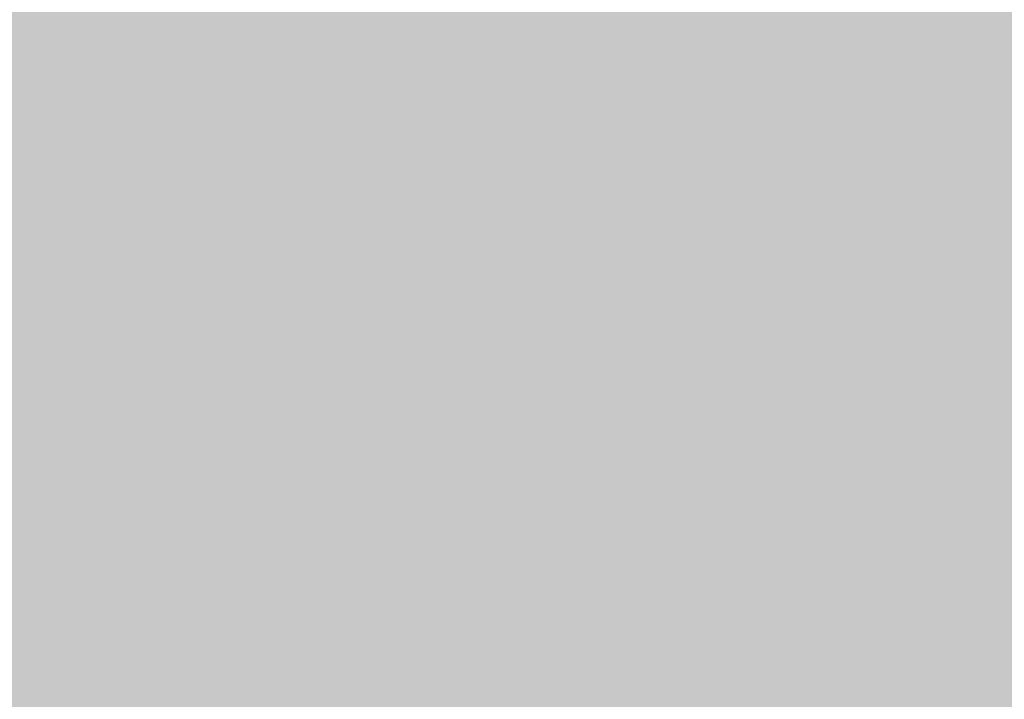
# Model space of a CAD drawing. Units: inches. Extents: x 2083 to 3317, y 1141 to 2115.
# Tile 38 of 256: x 2236.0667 to 2236.2151, y 1477.6562 to 1477.7587. Entities that reach past the tile are written whole.
import ezdxf

# ---------------------------------------------------------------- set-up
doc = ezdxf.new("R2010")
doc.units = ezdxf.units.IN
doc.layers.add('A-ANNO-DIMS', color=2, linetype='Continuous', lineweight=18)
doc.layers.add('A-WALL-PATT', color=251, linetype='Continuous', lineweight=13, true_color=0x636466)
doc.styles.get("Standard").update_dxf_attribs({"font": 'arial.ttf'})
doc.dimstyles.new('ISO-25', dxfattribs={"dimtxt": 12, "dimasz": 12, "dimexe": 1.25, "dimexo": 0.625, "dimtad": 1, "dimlunit": 3, "dimtxsty": 'Standard', "dimcen": 2.5, "dimadec": 0, "dimazin": 0, "dimtfac": 1, "dimtmove": 0, "dimatfit": 3, "dimfxl": 1, "dimarcsym": 0})

# ---------------------------------------------------------------- blocks, each defined once
blk = doc.blocks.new('*D30')
at = {"layer": 'A-ANNO-DIMS', "color": 0, "lineweight": -2, "transparency": 16777216}
for p, q in [((2240.01786, 1445.27381), (2240.01786, 1448.04553)), ((2254.32933, 1445.27381), (2254.32933, 1448.04553)), ((2228.01786, 1446.79553), (2216.01786, 1446.79553)), ((2240.01786, 1446.79553), (2254.32933, 1446.79553)), ((2266.32933, 1446.79553), (2413.76487, 1446.79553))]:
    blk.add_line(p, q, dxfattribs=at)
at = {"layer": 'A-ANNO-DIMS', "color": 0, "transparency": 16777216}
for points in [[(2228.01786, 1448.79553), (2228.01786, 1444.79553), (2240.01786, 1446.79553)], [(2266.32933, 1448.79553), (2266.32933, 1444.79553), (2254.32933, 1446.79553)]]:
    blk.add_solid(points, dxfattribs=at)
at = {"layer": 'Defpoints', "color": 0, "transparency": 16777216}
for p in [(2254.32933, 1446.79553), (2240.01786, 1444.64881), (2254.32933, 1444.64881)]:
    blk.add_point(p, dxfattribs=at)
at = {"layer": 'A-ANNO-DIMS', "color": 0, "transparency": 16777216, "insert": (2346.0471, 1453.62517), "char_height": 12, "attachment_point": 5}
blk.add_mtext('WC 1\'-2 1/2" TYP.', dxfattribs=at)
blk = doc.blocks.new('*D31')
at = {"layer": 'A-ANNO-DIMS', "color": 0, "lineweight": -2, "transparency": 16777216}
for p, q in [((2237.87114, 1456.64881), (2237.87114, 1541.91518)), ((2239.39286, 1444.64881), (2236.62114, 1444.64881)), ((2237.87114, 1431.54754), (2237.87114, 1444.64881)), ((2239.39286, 1431.54754), (2236.62114, 1431.54754)), ((2237.87114, 1419.54754), (2237.87114, 1407.54754))]:
    blk.add_line(p, q, dxfattribs=at)
at = {"layer": 'A-ANNO-DIMS', "color": 0, "transparency": 16777216}
for points in [[(2235.87114, 1456.64881), (2239.87114, 1456.64881), (2237.87114, 1444.64881)], [(2235.87114, 1419.54754), (2239.87114, 1419.54754), (2237.87114, 1431.54754)]]:
    blk.add_solid(points, dxfattribs=at)
at = {"layer": 'Defpoints', "color": 0, "transparency": 16777216}
for p in [(2237.87114, 1444.64881), (2240.01786, 1444.64881), (2240.01786, 1431.54754)]:
    blk.add_point(p, dxfattribs=at)
at = {"layer": 'A-ANNO-DIMS', "color": 0, "transparency": 16777216, "insert": (2231.21749, 1505.28199), "char_height": 12, "attachment_point": 5, "rotation": 90}
blk.add_mtext('1\'-1" TYP.', dxfattribs=at)
blk = doc.blocks.new('*D62')
at = {"layer": 'A-ANNO-DIMS', "color": 0, "lineweight": -2, "transparency": 16777216}
for p, q in [((2235.95978, 1469.38636), (2235.95978, 1522.36136)), ((2379.95978, 1469.38636), (2379.95978, 1522.36136)), ((2247.95978, 1521.11136), (2367.95978, 1521.11136))]:
    blk.add_line(p, q, dxfattribs=at)
at = {"layer": 'A-ANNO-DIMS', "color": 0, "transparency": 16777216}
for points in [[(2247.95978, 1523.11136), (2247.95978, 1519.11136), (2235.95978, 1521.11136)], [(2367.95978, 1523.11136), (2367.95978, 1519.11136), (2379.95978, 1521.11136)]]:
    blk.add_solid(points, dxfattribs=at)
at = {"layer": 'Defpoints', "color": 0, "transparency": 16777216}
for p in [(2379.95978, 1521.11136), (2235.95978, 1468.76136), (2379.95978, 1468.76136)]:
    blk.add_point(p, dxfattribs=at)
at = {"layer": 'A-ANNO-DIMS', "color": 0, "transparency": 16777216, "insert": (2307.95978, 1527.86324), "char_height": 12, "attachment_point": 5}
blk.add_mtext('12\'-0"', dxfattribs=at)

msp = doc.modelspace()

# ---------------------------------------------------------------- hatches: boundary and pattern name
at = {"layer": 'A-WALL-PATT'}
h = msp.add_hatch(color=256, dxfattribs=at)
h.dxf.hatch_style = 1
h.paths.add_polyline_path([(3126.95978, 2020.76136), (2748.95978, 2020.76136), (2604.95978, 2020.76136), (2226.95978, 2020.76136), (2226.95978, 1702.76136), (2466.95978, 1702.76136), (2466.95978, 1582.76136), (2418.95978, 1582.76136), (2418.95978, 1477.76136), (2226.95978, 1477.76136), (2226.95978, 1263.26136), (2544.95978, 1263.26136), (2544.95978, 1411.76136), (2604.95978, 1411.76136), (2685.95978, 1411.76136), (2685.95978, 1420.76136), (2604.95978, 1420.76136), (2604.95978, 1573.76136), (2604.95978, 1702.76136), (2604.95978, 2011.76136), (2748.95978, 2011.76136), (2748.95978, 1702.76136), (2862.95978, 1702.76136), (2862.95978, 1621.76136), (2871.95978, 1621.76136), (2871.95978, 1702.76136), (2883.95978, 1702.76136), (2883.95978, 1706.93946, -0.026459), (2883.95978, 1711.76136), (2757.95978, 1711.76136), (2757.95978, 1807.76136), (2787.95978, 1807.76136), (2787.95978, 1812.26136), (2757.95978, 1812.26136), (2757.95978, 2011.76136), (2877.95978, 2011.76136), (2877.95978, 1812.26136), (2847.95978, 1812.26136), (2847.95978, 1807.76136), (2889.83574, 1807.76136), (2889.83574, 1812.26136), (2882.45978, 1812.26136), (2882.45978, 2011.76136), (3117.95978, 2011.76136), (3117.95978, 1812.26136), (2937.83574, 1812.26136), (2937.83574, 1807.76136), (2995.70978, 1807.76136), (2995.70978, 1796.11767), (3000.20978, 1796.11767), (3000.20978, 1807.76136), (3117.95978, 1807.76136), (3117.95978, 1711.76136), (3000.20978, 1711.76136), (3000.20978, 1760.11767), (2998.5727, 1760.11767, -0.020711), (2995.70978, 1760.11767), (2995.70978, 1711.76136), (2931.95978, 1711.76136), (2931.95978, 1702.76136), (3126.95978, 1702.76136)])
h.paths.add_polyline_path([(2471.45978, 2011.76136), (2471.45978, 1810.01136), (2462.71694, 1810.01136), (2462.71694, 1805.51136), (2505.95978, 1805.51136), (2505.95978, 1810.01136), (2475.95978, 1810.01136), (2475.95978, 2011.76136), (2595.95978, 2011.76136), (2595.95978, 1810.01136), (2565.95978, 1810.01136), (2565.95978, 1805.51136), (2595.95978, 1805.51136), (2595.95978, 1711.76136), (2235.95978, 1711.76136), (2235.95978, 1805.51136), (2353.70978, 1805.51136), (2353.70978, 1796.05416), (2358.20978, 1796.05416), (2358.20978, 1805.51136), (2414.71694, 1805.51136), (2414.71694, 1810.01136), (2235.95978, 1810.01136), (2235.95978, 2011.76136)], flags=16)
h.paths.add_polyline_path([(2270.20473, 1994.61001), (2270.20473, 1970.61001), (2246.20473, 1970.61001), (2246.20473, 1994.61001)], flags=0)
edge = h.paths.add_edge_path(flags=0)
edge.add_ellipse((2332.02739, 1899.79818), major_axis=(-3.04299, 3.04299), ratio=0.1682525, start_angle=-161.33217, end_angle=-156.30711, ccw=False)
edge.add_ellipse((2333.08204, 1898.74353), major_axis=(-1.05465, 1.05465), ratio=0.4535321, start_angle=-123.37102, end_angle=-94.15911)
edge = h.paths.add_edge_path(flags=0)
edge.add_ellipse((2332.02739, 1968.87629), major_axis=(3.04299, 3.04299), ratio=0.1682525, start_angle=18.66783, end_angle=23.69289)
edge.add_spline(control_points=[(2332.9256, 1970.6911), (2332.22677, 1970.3361), (2330.89371, 1969.65891), (2328.41308, 1970.93214), (2327.20393, 1967.74871), (2324.7096, 1969.95559), (2322.53282, 1967.01235), (2320.01285, 1971.29581), (2317.68031, 1968.15784), (2316.04053, 1967.10205), (2315.4269, 1966.8096)], knot_values=[0, 0, 0, 0, 2.267059, 4.324559, 6.685584, 8.878641, 11.121502, 14.300359, 17.755284, 19.732645, 19.732645, 19.732645, 19.732645], degree=3, periodic=0)
edge.add_ellipse((2332.02739, 1968.87629), major_axis=(3.04299, 3.04299), ratio=0.1682525, start_angle=18.66783, end_angle=23.69289, ccw=False)
edge.add_ellipse((2333.08204, 1969.93094), major_axis=(1.05465, 1.05465), ratio=0.4535321, start_angle=56.62898, end_angle=85.84089, ccw=False)
edge = h.paths.add_edge_path(flags=0)
edge.add_spline(control_points=[(2296.42829, 1967.98791), (2293.6278, 1965.33631), (2287.70362, 1959.72709), (2299.74386, 1949.9957), (2294.53259, 1935.66853), (2290.57323, 1920.60351), (2293.39412, 1909.97369), (2296.18541, 1904.96654)], knot_values=[0.099185, 0.099185, 0.099185, 0.099185, 0.345301, 0.619822, 0.982653, 1.386093, 1.810555, 1.810555, 1.810555, 1.810555], degree=3, periodic=0)
edge.add_spline(control_points=[(2296.18541, 1904.96654), (2297.38358, 1902.6193), (2298.00097, 1901.94931), (2298.55297, 1901.46815)], knot_values=[0.006246, 0.006246, 0.006246, 0.006246, 0.055476, 0.055476, 0.055476, 0.055476], degree=3, periodic=0)
edge.add_spline(control_points=[(2298.55297, 1901.46815), (2297.25861, 1900.92322), (2295.22529, 1900.23213), (2293.06023, 1900.61421), (2292.10142, 1900.78841), (2292.08958, 1900.79057)], knot_values=[0.312835, 0.312835, 0.312835, 0.312835, 0.40178, 0.474987, 0.475903, 0.475903, 0.475903, 0.475903], degree=3, periodic=0)
edge.add_arc((2292.79365, 1904.66411), 3.93701, 215.4209, 259.69818, ccw=False)
edge.add_spline(control_points=[(2289.58531, 1902.3823), (2289.47665, 1902.53509), (2289.36848, 1902.68804), (2289.26086, 1902.84117)], knot_values=[0.102872, 0.102872, 0.102872, 0.102872, 0.116896, 0.116896, 0.116896, 0.116896], degree=3, periodic=0)
edge.add_spline(control_points=[(2289.26086, 1902.84117), (2288.6866, 1902.55019), (2287.64005, 1902.0199), (2285.88134, 1901.87395), (2283.85297, 1901.50435), (2281.71999, 1899.71054), (2278.46699, 1899.49294), (2276.15714, 1901.8832), (2272.25895, 1899.80407), (2267.77761, 1901.84318), (2262.24388, 1900.18403), (2257.41493, 1901.78206), (2254.31837, 1900.72612), (2253.17828, 1900.33734)], knot_values=[0, 0, 0, 0, 1.907977, 3.477176, 5.261074, 7.972851, 11.680248, 13.717921, 16.939592, 22.789562, 27.502503, 33.595215, 37.145618, 37.145618, 37.145618, 37.145618], degree=3, periodic=0)
edge.add_line((2253.17828, 1900.33734), (2250.24424, 1902.84117))
edge.add_line((2250.24424, 1902.84117), (2250.24424, 1965.8333))
edge.add_line((2250.24424, 1965.8333), (2253.17828, 1968.33712))
edge.add_spline(control_points=[(2253.17828, 1968.33712), (2254.31837, 1967.94835), (2257.41493, 1966.89241), (2262.24388, 1968.49043), (2267.77761, 1966.83128), (2271.52673, 1968.53722), (2273.87591, 1967.82829), (2274.2067, 1967.72764)], knot_values=[0, 0, 0, 0, 0.09018, 0.244935, 0.364644, 0.513233, 0.537855, 0.537855, 0.537855, 0.537855], degree=3, periodic=0)
edge.add_arc((2274.35289, 1963.79335), 3.93701, 72.05113, 92.12795, ccw=False)
edge.add_arc((2281.29693, 1985.23), 18.5963, 252.051134, 288.565722)
edge.add_arc((2292.31672, 1956.02888), 12.64608, 71.026788, 113.778218, ccw=False)
edge = h.paths.add_edge_path(flags=0)
edge.add_spline(control_points=[(2274.89941, 1951.85619), (2275.06616, 1951.61659), (2275.23269, 1951.37659), (2275.39799, 1951.13585)], knot_values=[1.409916, 1.409916, 1.409916, 1.409916, 1.43159, 1.43159, 1.43159, 1.43159], degree=3, periodic=0)
edge.add_spline(control_points=[(2275.39799, 1951.13585), (2275.79211, 1950.56189), (2276.17923, 1949.98377), (2276.54555, 1949.3971)], knot_values=[1.358238, 1.358238, 1.358238, 1.358238, 1.409916, 1.409916, 1.409916, 1.409916], degree=3, periodic=0)
edge.add_line((2276.54555, 1949.3971), (2277.43729, 1947.86218))
edge.add_spline(control_points=[(2277.43729, 1947.86218), (2276.30383, 1945.67311), (2274.6397, 1942.42688), (2274.63161, 1938.0939), (2272.79912, 1930.85155), (2274.35643, 1943.89705), (2275.94768, 1947.92336), (2276.54555, 1949.3971)], knot_values=[0.005632, 0.005632, 0.005632, 0.005632, 0.186014, 0.266002, 0.357087, 0.59639, 0.739732, 0.739732, 0.739732, 0.739732], degree=3, periodic=0)
edge.add_spline(control_points=[(2276.54555, 1949.3971), (2276.17923, 1949.98377), (2275.79211, 1950.56189), (2275.39799, 1951.13585)], knot_values=[1.358238, 1.358238, 1.358238, 1.358238, 1.409916, 1.409916, 1.409916, 1.409916], degree=3, periodic=0)
edge.add_spline(control_points=[(2275.39799, 1951.13585), (2274.9425, 1950.08045), (2274.20776, 1948.02527), (2273.9346, 1944.85148), (2272.46853, 1937.62749), (2273.46622, 1945.69647), (2274.70062, 1951.05947), (2274.89941, 1951.85619)], knot_values=[0.104364, 0.104364, 0.104364, 0.104364, 0.189636, 0.269624, 0.36071, 0.600013, 0.644622, 0.644622, 0.644622, 0.644622], degree=3, periodic=0)
h.paths.add_polyline_path([(2269.16751, 1963.12757, -0.357527), (2268.17063, 1960.97637, -0.092561), (2268.17063, 1939.43632, -0.357527), (2269.16751, 1937.28512, -0.357527), (2267.01631, 1938.282, -0.164785), (2254.68558, 1938.282, -0.357527), (2252.53438, 1937.28512, -0.357527), (2253.53126, 1939.43632, -0.092561), (2253.53126, 1960.97637, -0.357527), (2252.53438, 1963.12757, -0.357527), (2254.68558, 1962.13069, -0.164785), (2267.01631, 1962.13069, -0.357527)], flags=0)
h.paths.add_polyline_path([(2248.87407, 1967.8018), (2248.87407, 1957.02771), (2249.45778, 1957.02771), (2249.45778, 1911.64676), (2248.87407, 1911.64676), (2248.87407, 1900.87267), (2246.51186, 1900.87267, 0.197327), (2244.14966, 1902.45687), (2244.14966, 1966.21759, 0.197327), (2246.51186, 1967.8018)], flags=0)
h.paths.add_polyline_path([(2269.16751, 1931.38934, -0.357527), (2268.17063, 1929.23814, -0.092561), (2268.17063, 1907.6981, -0.357527), (2269.16751, 1905.54689, -0.357527), (2267.01631, 1906.54377, -0.164785), (2254.68558, 1906.54377, -0.357527), (2252.53438, 1905.54689, -0.357527), (2253.53126, 1907.6981, -0.092561), (2253.53126, 1929.23814, -0.357527), (2252.53438, 1931.38934, -0.357527), (2254.68558, 1930.39246, -0.164785), (2267.01631, 1930.39246, -0.357527)], flags=0)
edge = h.paths.add_edge_path(flags=0)
edge.add_spline(control_points=[(2276.19686, 1906.7237), (2276.16814, 1909.02893), (2276.11405, 1913.37185), (2270.59842, 1924.92498), (2273.90517, 1919.01278), (2275.92171, 1916.26206), (2275.47457, 1912.40215), (2277.25787, 1910.38062), (2276.69604, 1908.22504), (2276.64622, 1906.81302), (2276.61782, 1906.00841)], knot_values=[0, 0, 0, 0, 8.61026, 16.221274, 18.843057, 23.804898, 27.440828, 29.356102, 31.203478, 33.650687, 33.650687, 33.650687, 33.650687], degree=3, periodic=0)
edge.add_spline(control_points=[(2276.61782, 1906.00841), (2276.62331, 1905.62414), (2276.49774, 1904.62866), (2275.44178, 1903.85473), (2274.93731, 1903.08045), (2274.85908, 1902.84117)], knot_values=[0.156488, 0.156488, 0.156488, 0.156488, 0.184398, 0.231376, 0.250598, 0.250598, 0.250598, 0.250598], degree=3, periodic=0)
edge.add_line((2274.85908, 1902.84117), (2276.50598, 1902.84117))
edge.add_spline(control_points=[(2276.50598, 1902.84117), (2276.78831, 1903.08494), (2277.66507, 1904.1252), (2278.24954, 1904.34074), (2277.65387, 1908.52739), (2278.15567, 1906.22781), (2278.10046, 1905.28595), (2278.84667, 1904.06901), (2277.85679, 1903.41495), (2277.87419, 1902.99105), (2277.90356, 1902.84117)], knot_values=[0.059574, 0.059574, 0.059574, 0.059574, 0.080753, 0.103741, 0.16972, 0.176036, 0.207137, 0.240474, 0.262341, 0.27366, 0.27366, 0.27366, 0.27366], degree=3, periodic=0)
edge.add_line((2277.90356, 1902.84117), (2280.02983, 1902.84117))
edge.add_spline(control_points=[(2280.02983, 1902.84117), (2279.88822, 1903.0884), (2279.49926, 1903.98155), (2280.15228, 1905.93935), (2278.10362, 1909.65776), (2279.76239, 1907.18529), (2280.3279, 1904.87486), (2280.48511, 1903.48959), (2281.46327, 1903.24943), (2281.75834, 1902.9365), (2281.83404, 1902.84117)], knot_values=[0.013856, 0.013856, 0.013856, 0.013856, 0.034874, 0.088867, 0.107879, 0.126738, 0.158714, 0.193757, 0.217487, 0.226722, 0.226722, 0.226722, 0.226722], degree=3, periodic=0)
edge.add_spline(control_points=[(2281.83404, 1902.84117), (2281.78753, 1902.8267), (2281.64702, 1902.78299), (2281.39553, 1902.85949), (2281.08808, 1902.98524), (2280.72068, 1903.0609), (2280.33345, 1903.02573), (2280.12477, 1902.89888), (2280.02983, 1902.84117)], knot_values=[0, 0, 0, 0, 0.14413, 0.435517, 0.749276, 1.153046, 1.548371, 1.878348, 1.878348, 1.878348, 1.878348], degree=3, periodic=0)
edge.add_line((2280.02983, 1902.84117), (2277.90356, 1902.84117))
edge.add_spline(control_points=[(2277.90356, 1902.84117), (2277.89286, 1902.79586), (2277.8654, 1902.67964), (2277.60748, 1902.68748), (2277.27405, 1902.8007), (2276.83792, 1902.61977), (2276.58381, 1902.78926), (2276.50598, 1902.84117)], knot_values=[0, 0, 0, 0, 0.127189, 0.326199, 0.628009, 1.24357, 1.515331, 1.515331, 1.515331, 1.515331], degree=3, periodic=0)
edge.add_line((2276.50598, 1902.84117), (2274.85908, 1902.84117))
edge.add_spline(control_points=[(2274.85908, 1902.84117), (2274.81444, 1902.89859), (2274.72513, 1903.01345), (2274.49348, 1903.11897), (2274.24429, 1902.96054), (2273.93712, 1903.18494), (2273.61404, 1902.98314), (2273.40832, 1902.88304), (2273.32225, 1902.84117)], knot_values=[0, 0, 0, 0, 0.21843, 0.436957, 0.687977, 0.990379, 1.398396, 1.69185, 1.69185, 1.69185, 1.69185], degree=3, periodic=0)
edge.add_spline(control_points=[(2273.32225, 1902.84117), (2273.61674, 1903.44569), (2274.274, 1904.53825), (2276.02724, 1904.5737), (2276.20696, 1906.58364), (2276.19686, 1906.7237)], knot_values=[0.012227, 0.012227, 0.012227, 0.012227, 0.059472, 0.106218, 0.134458, 0.134458, 0.134458, 0.134458], degree=3, periodic=0)
h.paths.add_polyline_path([(2270.77605, 1897.78983), (2270.77605, 1873.78983), (2246.77605, 1873.78983), (2246.77605, 1897.78983)], flags=0)
h.paths.add_polyline_path([(2353.70978, 1760.00506), (2353.70978, 1760.05416), (2358.20978, 1760.05416, -0.033729)], flags=0)
h.paths.add_polyline_path([(2321.81912, 1737.52919), (2341.99533, 1737.52919, -0.414214), (2343.20327, 1736.32124), (2343.20327, 1721.0206, -0.414214), (2341.99533, 1719.81265), (2321.81912, 1719.81265, -0.414214), (2320.61117, 1721.0206), (2320.61117, 1736.32124, -0.414214)], flags=0)
h.paths.add_polyline_path([(2324.23501, 1736.32124), (2339.57944, 1736.32124, -0.414214), (2341.99533, 1733.90535), (2341.99533, 1725.44973, -0.414214), (2339.57944, 1723.03384), (2333.68059, 1723.03384), (2333.84532, 1722.04547, -0.870646), (2335.4254, 1721.82589, -0.767327), (2333.92269, 1721.42324), (2331.29102, 1721.42324, -0.767327), (2329.78832, 1721.82589, -0.870646), (2331.3684, 1722.04547), (2331.53313, 1723.03384), (2324.23501, 1723.03384, -0.414214), (2321.81912, 1725.44973), (2321.81912, 1733.90535, -0.414214)], flags=0)
h.paths.add_polyline_path([(2570.48379, 1928.61544), (2589.68379, 1928.61544), (2590.16883, 1928.61544), (2590.16883, 1904.9934), (2570.48379, 1904.9934)], flags=0)
h.paths.add_polyline_path([(2574.44732, 1927.26382, -1), (2572.82884, 1927.26382, -1)], flags=0)
h.paths.add_polyline_path([(2573.08987, 1926.94088), (2573.92503, 1927.77604), (2574.14774, 1927.55333), (2573.31258, 1926.71817)], flags=0)
h.paths.add_polyline_path([(2578.77906, 1919.72962, -1), (2571.59166, 1919.72962, -1)], flags=0)
h.paths.add_polyline_path([(2578.38536, 1919.72962, -1), (2571.98536, 1919.72962, -1)], flags=0)
h.paths.add_polyline_path([(2331.59576, 1729.47622, -1), (2333.61795, 1729.47622, -1)], flags=0)
h.paths.add_polyline_path([(2578.03423, 1927.26382, -1), (2576.41574, 1927.26382, -1)], flags=0)
h.paths.add_polyline_path([(2576.68885, 1927.53109), (2576.91156, 1927.7538), (2577.74673, 1926.91863), (2577.52402, 1926.69592)], flags=0)
h.paths.add_polyline_path([(2578.13906, 1909.85954, -1), (2572.23166, 1909.85954, -1)], flags=0)
h.paths.add_polyline_path([(2577.74536, 1909.85954, -1), (2572.62536, 1909.85954, -1)], flags=0)
h.paths.add_polyline_path([(2583.79772, 1927.26382, -1), (2582.17923, 1927.26382, -1)], flags=0)
h.paths.add_polyline_path([(2582.71865, 1927.7538), (2583.55381, 1926.91863), (2583.3311, 1926.69592), (2582.49594, 1927.53109)], flags=0)
h.paths.add_polyline_path([(2582.49594, 1927.53109), (2582.71865, 1927.7538), (2583.55381, 1926.91863), (2583.3311, 1926.69592)], flags=0)
h.paths.add_polyline_path([(2587.73906, 1920.52962, -1), (2581.83166, 1920.52962, -1)], flags=0)
h.paths.add_polyline_path([(2587.34536, 1920.52962, -1), (2582.22536, 1920.52962, -1)], flags=0)
h.paths.add_polyline_path([(2587.38462, 1927.26382, -1), (2585.76613, 1927.26382, -1)], flags=0)
h.paths.add_polyline_path([(2586.08199, 1926.98025), (2586.91716, 1927.81541), (2587.13987, 1927.5927), (2586.3047, 1926.75754)], flags=0)
h.paths.add_polyline_path([(2588.37906, 1910.65954, -1), (2581.19166, 1910.65954, -1)], flags=0)
h.paths.add_polyline_path([(2587.98536, 1910.65954, -1), (2581.58536, 1910.65954, -1)], flags=0)
h.paths.add_polyline_path([(2417.16773, 1729.4779), (2437.34394, 1729.4779, -0.414214), (2438.55188, 1728.26995), (2438.55188, 1712.96931, -0.414214), (2437.34394, 1711.76136), (2417.16773, 1711.76136, -0.414214), (2415.95978, 1712.96931), (2415.95978, 1728.26995, -0.414214)], flags=0)
h.paths.add_polyline_path([(2419.58362, 1728.26995), (2434.92805, 1728.26995, -0.414214), (2437.34394, 1725.85406), (2437.34394, 1717.39844, -0.414214), (2434.92805, 1714.98255), (2429.0292, 1714.98255), (2429.19393, 1713.99418, -0.870646), (2430.77401, 1713.7746, -0.767327), (2429.2713, 1713.37195), (2426.63963, 1713.37195, -0.767327), (2425.13693, 1713.7746, -0.870646), (2426.71701, 1713.99418), (2426.88174, 1714.98255), (2419.58362, 1714.98255, -0.414214), (2417.16773, 1717.39844), (2417.16773, 1725.85406, -0.414214)], flags=0)
h.paths.add_polyline_path([(2419.58362, 1728.26995), (2434.92805, 1728.26995, -0.414214), (2437.34394, 1725.85406), (2437.34394, 1717.39844, -0.414214), (2434.92805, 1714.98255), (2429.0292, 1714.98255), (2428.35812, 1719.00903), (2427.55282, 1719.00903), (2426.88174, 1714.98255), (2419.58362, 1714.98255, -0.414214), (2417.16773, 1717.39844), (2417.16773, 1725.85406, -0.414214)], flags=0)
h.paths.add_polyline_path([(2426.94437, 1721.42492, -1), (2428.96656, 1721.42492, -1)], flags=0)
h.paths.add_polyline_path([(2475.95978, 1702.76136), (2595.95978, 1702.76136), (2595.95978, 1582.76136), (2475.95978, 1582.76136)], flags=16)
h.paths.add_polyline_path([(2427.95978, 1573.76136), (2595.95978, 1573.76136), (2595.95978, 1468.76136), (2595.95978, 1420.76136), (2384.45978, 1420.76136), (2384.45978, 1468.76136), (2427.95978, 1468.76136)], flags=16)
h.paths.add_polyline_path([(2379.95978, 1468.76136), (2379.95978, 1420.76136), (2235.95978, 1420.76136), (2235.95978, 1468.76136)], flags=16)
h.paths.add_polyline_path([(2317.816, 1466.69577), (2337.9922, 1466.69577, -0.414214), (2339.20015, 1465.48782), (2339.20015, 1450.18718, -0.414214), (2337.9922, 1448.97923), (2317.816, 1448.97923, -0.414214), (2316.60805, 1450.18718), (2316.60805, 1465.48782, -0.414214)], flags=0)
h.paths.add_polyline_path([(2320.23189, 1465.48782), (2335.57631, 1465.48782, -0.414214), (2337.9922, 1463.07193), (2337.9922, 1454.61631, -0.414214), (2335.57631, 1452.20042), (2329.67747, 1452.20042), (2329.84219, 1451.21205, -0.870646), (2331.42228, 1450.99247, -0.767327), (2329.91957, 1450.58983), (2327.2879, 1450.58983, -0.767327), (2325.7852, 1450.99247, -0.870646), (2327.36528, 1451.21205), (2327.53001, 1452.20042), (2320.23189, 1452.20042, -0.414214), (2317.816, 1454.61631), (2317.816, 1463.07193, -0.414214)], flags=0)
h.paths.add_polyline_path([(2320.23189, 1465.48782), (2335.57631, 1465.48782, -0.414214), (2337.9922, 1463.07193), (2337.9922, 1454.61631, -0.414214), (2335.57631, 1452.20042), (2329.67747, 1452.20042), (2329.00638, 1456.22691), (2328.20109, 1456.22691), (2327.53001, 1452.20042), (2320.23189, 1452.20042, -0.414214), (2317.816, 1454.61631), (2317.816, 1463.07193, -0.414214)], flags=0)
h.paths.add_polyline_path([(2327.59264, 1458.6428, -1), (2329.61483, 1458.6428, -1)], flags=0)
h.paths.add_polyline_path([(2244.41174, 1433.34045), (2241.92094, 1433.34045, -0.414214), (2240.01786, 1435.24354), (2240.01786, 1440.95281, -0.414211), (2241.92093, 1442.8559), (2244.41174, 1442.8559, -1.976472)], flags=0)
h.paths.add_polyline_path([(2245.35689, 1434.39754, -0.414214), (2245.35689, 1441.79881, -2.144098)], flags=0)
h.paths.add_polyline_path([(2535.95978, 1416.26136), (2535.95978, 1272.26136), (2235.95978, 1272.26136), (2235.95978, 1416.26136)], flags=16)
h.paths.add_polyline_path([(2260.11956, 1384.29284), (2260.11956, 1362.03865), (2237.86537, 1362.03865), (2237.86537, 1384.29284)], flags=0)
edge = h.paths.add_edge_path(flags=0)
edge.add_line((2318.25185, 1362.0933), (2318.1458, 1362.00097))
edge.add_ellipse((2317.44512, 1360.43104), major_axis=(2.82164, 2.82164), ratio=0.1682525, start_angle=18.66783, end_angle=20.94813, ccw=False)
edge.add_ellipse((2318.42305, 1361.40897), major_axis=(0.97793, 0.97793), ratio=0.4535321, start_angle=56.62898, end_angle=70.2262, ccw=False)
edge = h.paths.add_edge_path(flags=0)
edge.add_line((2319.10737, 1295.57108), (2319.01504, 1295.67713))
edge.add_ellipse((2317.44512, 1296.37781), major_axis=(-2.82164, 2.82164), ratio=0.1682525, start_angle=-161.33217, end_angle=-159.05187, ccw=False)
edge.add_ellipse((2318.42305, 1295.39988), major_axis=(-0.97793, 0.97793), ratio=0.4535321, start_angle=-123.37102, end_angle=-109.7738)
edge = h.paths.add_edge_path(flags=0)
edge.add_spline(control_points=[(2284.21035, 1301.17022), (2284.58069, 1300.44472), (2284.89119, 1299.89202), (2285.15955, 1299.46102)], knot_values=[0.039066, 0.039066, 0.039066, 0.039066, 0.055476, 0.055476, 0.055476, 0.055476], degree=3, periodic=0)
edge.add_line((2285.15955, 1299.46102), (2284.21035, 1301.17022))
edge = h.paths.add_edge_path(flags=0)
edge.add_line((2280.41246, 1297.29801), (2283.36999, 1297.03612))
edge.add_line((2283.36999, 1297.03612), (2286.40569, 1297.92631))
edge.add_spline(control_points=[(2286.40569, 1297.92631), (2285.30549, 1297.46312), (2284.34478, 1297.12915), (2283.36999, 1297.03612)], knot_values=[0.394369, 0.394369, 0.394369, 0.394369, 0.475903, 0.475903, 0.475903, 0.475903], degree=3, periodic=0)
edge.add_spline(control_points=[(2283.36999, 1297.03612), (2283.28139, 1297.02767), (2282.31629, 1296.95734), (2281.3125, 1297.13448), (2280.42344, 1297.29602), (2280.41246, 1297.29801)], knot_values=[0.312835, 0.312835, 0.312835, 0.312835, 0.320246, 0.393453, 0.394369, 0.394369, 0.394369, 0.394369], degree=3, periodic=0)
edge = h.paths.add_edge_path(flags=0)
edge.add_line((2284.43556, 1359.60729), (2280.44629, 1355.32805))
edge.add_line((2280.44629, 1355.32805), (2279.57999, 1351.01775))
edge.add_line((2279.57999, 1351.01775), (2282.41297, 1346.58043))
edge.add_spline(control_points=[(2282.41297, 1346.58043), (2283.15333, 1345.58924), (2284.2529, 1344.0289), (2284.80104, 1342.38717), (2284.93516, 1341.80554)], knot_values=[1.240098, 1.240098, 1.240098, 1.240098, 1.332892, 1.382712, 1.382712, 1.382712, 1.382712], degree=3, periodic=0)
edge.add_spline(control_points=[(2284.93516, 1341.80554), (2285.31911, 1340.1406), (2285.23303, 1338.4092), (2284.90994, 1336.65412)], knot_values=[1.097484, 1.097484, 1.097484, 1.097484, 1.240098, 1.240098, 1.240098, 1.240098], degree=3, periodic=0)
edge.add_spline(control_points=[(2284.90994, 1336.65412), (2284.58685, 1334.89904), (2284.02675, 1333.12027), (2283.46264, 1331.36058)], knot_values=[0.95487, 0.95487, 0.95487, 0.95487, 1.097484, 1.097484, 1.097484, 1.097484], degree=3, periodic=0)
edge.add_line((2283.46264, 1331.36058), (2281.89038, 1326.15336))
edge.add_line((2281.89038, 1326.15336), (2280.75626, 1321.05609))
edge.add_line((2280.75626, 1321.05609), (2280.2992, 1316.00198))
edge.add_line((2280.2992, 1316.00198), (2280.71593, 1310.95007))
edge.add_line((2280.71593, 1310.95007), (2282.02809, 1305.97214))
edge.add_line((2282.02809, 1305.97214), (2284.21035, 1301.17022))
edge.add_spline(control_points=[(2284.21035, 1301.17022), (2283.34073, 1302.73019), (2282.6119, 1304.33649), (2282.02809, 1305.97214)], knot_values=[0.099185, 0.099185, 0.099185, 0.099185, 0.241799, 0.241799, 0.241799, 0.241799], degree=3, periodic=0)
edge.add_spline(control_points=[(2282.02809, 1305.97214), (2281.44428, 1307.60778), (2281.00549, 1309.27276), (2280.71593, 1310.95007)], knot_values=[0.241799, 0.241799, 0.241799, 0.241799, 0.384413, 0.384413, 0.384413, 0.384413], degree=3, periodic=0)
edge.add_spline(control_points=[(2280.71593, 1310.95007), (2280.43324, 1312.58761), (2280.28939, 1314.27696), (2280.29889, 1315.96203), (2280.2992, 1316.00198)], knot_values=[0.384413, 0.384413, 0.384413, 0.384413, 0.523647, 0.527028, 0.527028, 0.527028, 0.527028], degree=3, periodic=0)
edge.add_spline(control_points=[(2280.2992, 1316.00198), (2280.31233, 1317.68696), (2280.47787, 1319.36793), (2280.75626, 1321.05609)], knot_values=[0.527028, 0.527028, 0.527028, 0.527028, 0.669642, 0.669642, 0.669642, 0.669642], degree=3, periodic=0)
edge.add_spline(control_points=[(2280.75626, 1321.05609), (2281.03465, 1322.74425), (2281.42588, 1324.43961), (2281.89038, 1326.15336)], knot_values=[0.669642, 0.669642, 0.669642, 0.669642, 0.812256, 0.812256, 0.812256, 0.812256], degree=3, periodic=0)
edge.add_spline(control_points=[(2281.89038, 1326.15336), (2282.26438, 1327.53325), (2282.78787, 1329.26181), (2283.35275, 1331.01778), (2283.46264, 1331.36058)], knot_values=[0.812256, 0.812256, 0.812256, 0.812256, 0.927087, 0.95487, 0.95487, 0.95487, 0.95487], degree=3, periodic=0)
edge.add_line((2283.46264, 1331.36058), (2284.90994, 1336.65412))
edge.add_line((2284.90994, 1336.65412), (2284.93516, 1341.80554))
edge.add_line((2284.93516, 1341.80554), (2282.41297, 1346.58043))
edge.add_spline(control_points=[(2282.41297, 1346.58043), (2281.27513, 1348.10379), (2280.07845, 1349.57032), (2279.57999, 1351.01775)], knot_values=[1.382712, 1.382712, 1.382712, 1.382712, 1.525326, 1.525326, 1.525326, 1.525326], degree=3, periodic=0)
edge.add_spline(control_points=[(2279.57999, 1351.01775), (2279.44328, 1351.41472), (2279.13631, 1352.85692), (2279.73519, 1354.29039), (2280.44629, 1355.32805)], knot_values=[1.525326, 1.525326, 1.525326, 1.525326, 1.564439, 1.667941, 1.667941, 1.667941, 1.667941], degree=3, periodic=0)
edge.add_spline(control_points=[(2280.44629, 1355.32805), (2281.42611, 1356.75784), (2282.93084, 1358.18256), (2284.43556, 1359.60729)], knot_values=[1.667941, 1.667941, 1.667941, 1.667941, 1.810555, 1.810555, 1.810555, 1.810555], degree=3, periodic=0)
edge.add_arc((2280.62307, 1348.51818), 11.72618, 71.026788, 113.778218)
edge.add_arc((2270.40489, 1375.59516), 17.24357, 252.051134, 288.565722, ccw=False)
edge.add_arc((2263.96597, 1355.71785), 3.65062, 72.05113, 92.12795)
edge.add_arc((2263.96597, 1355.71785), 3.65062, 92.12795, 177.98513)
edge.add_spline(control_points=[(2260.3176, 1355.8462), (2260.26042, 1354.22067), (2260.55128, 1350.18655), (2262.99934, 1346.76625), (2264.47274, 1344.64902)], knot_values=[1.43159, 1.43159, 1.43159, 1.43159, 1.564144, 1.770695, 1.770695, 1.770695, 1.770695], degree=3, periodic=0)
edge.add_line((2264.47274, 1344.64902), (2264.93559, 1343.98253))
edge.add_spline(control_points=[(2263.80104, 1340.24811), (2263.84324, 1340.51409), (2264.06724, 1341.75647), (2264.51269, 1343.00245), (2264.93505, 1343.98108)], knot_values=[0.53657, 0.53657, 0.53657, 0.53657, 0.559349, 0.644622, 0.644622, 0.644622, 0.644622], degree=3, periodic=0)
edge.add_spline(control_points=[(2264.93505, 1343.98108), (2265.11777, 1343.71497), (2265.29888, 1343.44791), (2265.47676, 1343.17936)], knot_values=[1.384077, 1.384077, 1.384077, 1.384077, 1.409916, 1.409916, 1.409916, 1.409916], degree=3, periodic=0)
edge.add_spline(control_points=[(2265.47676, 1343.17936), (2265.65464, 1342.91082), (2265.8293, 1342.64081), (2265.99913, 1342.36881)], knot_values=[1.358238, 1.358238, 1.358238, 1.358238, 1.384077, 1.384077, 1.384077, 1.384077], degree=3, periodic=0)
edge.add_line((2265.99913, 1342.36881), (2266.82601, 1340.94555))
edge.add_spline(control_points=[(2266.82601, 1340.94555), (2268.8944, 1337.08969), (2271.39817, 1325.843), (2270.51616, 1310.56856), (2275.91938, 1301.86061), (2277.78951, 1299.19945)], knot_values=[0.116896, 0.116896, 0.116896, 0.116896, 0.472987, 1.050969, 1.313793, 1.313793, 1.313793, 1.313793], degree=3, periodic=0)
edge.add_spline(control_points=[(2277.78951, 1299.19945), (2277.83941, 1299.12845), (2277.88943, 1299.0575), (2277.93957, 1298.98658)], knot_values=[0.109884, 0.109884, 0.109884, 0.109884, 0.116896, 0.116896, 0.116896, 0.116896], degree=3, periodic=0)
edge.add_line((2277.93957, 1298.98658), (2277.78885, 1299.19911))
edge.add_spline(control_points=[(2277.78885, 1299.19911), (2277.25658, 1298.92941), (2276.28635, 1298.4379), (2275.03935, 1298.33442), (2274.38333, 1298.2389), (2274.21525, 1298.20934)], knot_values=[33.12187, 33.12187, 33.12187, 33.12187, 35.029056, 36.598255, 37.144827, 37.144827, 37.144827, 37.144827], degree=3, periodic=0)
edge.add_line((2274.21525, 1298.20934), (2273.07315, 1297.89296))
edge.add_spline(control_points=[(2273.07315, 1297.89296), (2272.32294, 1297.57978), (2271.03915, 1296.51051), (2269.24839, 1296.22606), (2268.4231, 1296.37465)], knot_values=[26.532584, 26.532584, 26.532584, 26.532584, 29.198919, 31.839101, 31.839101, 31.839101, 31.839101], degree=3, periodic=0)
edge.add_line((2268.4231, 1296.37465), (2263.8785, 1297.45753))
edge.add_spline(control_points=[(2263.8785, 1297.45753), (2263.55608, 1297.35943), (2261.86031, 1296.83869), (2260.23878, 1297.28241), (2258.93345, 1297.51646)], knot_values=[15.919551, 15.919551, 15.919551, 15.919551, 16.939592, 21.226067, 21.226067, 21.226067, 21.226067], degree=3, periodic=0)
edge.add_line((2258.93345, 1297.51646), (2254.05523, 1297.32901))
edge.add_spline(control_points=[(2254.05523, 1297.32901), (2253.75553, 1297.29582), (2252.11368, 1297.16517), (2250.46187, 1297.54422), (2249.12969, 1297.66788)], knot_values=[5.306517, 5.306517, 5.306517, 5.306517, 6.276435, 10.613034, 10.613034, 10.613034, 10.613034], degree=3, periodic=0)
edge.add_line((2249.12969, 1297.66788), (2244.33165, 1296.87776))
edge.add_line((2244.33165, 1296.87776), (2241.61103, 1299.19945))
edge.add_line((2241.61103, 1299.19945), (2241.61103, 1357.6094))
edge.add_line((2241.61103, 1357.6094), (2244.33165, 1359.9311))
edge.add_line((2244.33165, 1359.9311), (2252.72882, 1359.54269))
edge.add_spline(control_points=[(2252.72882, 1359.54269), (2252.87094, 1359.54644), (2253.30574, 1359.54817), (2253.73984, 1359.51427), (2254.03174, 1359.48243)], knot_values=[0.233291, 0.233291, 0.233291, 0.233291, 0.244935, 0.268927, 0.268927, 0.268927, 0.268927], degree=3, periodic=0)
edge.add_line((2254.03174, 1359.48243), (2259.58719, 1359.41639))
edge.add_spline(control_points=[(2259.58719, 1359.41639), (2260.67707, 1359.6285), (2262.0732, 1359.897), (2263.52369, 1359.45928), (2263.83042, 1359.36595)], knot_values=[0.422516, 0.422516, 0.422516, 0.422516, 0.513233, 0.537855, 0.537855, 0.537855, 0.537855], degree=3, periodic=0)
edge.add_arc((2263.96597, 1355.71785), 3.65062, 72.05113, 92.12795, ccw=False)
edge.add_arc((2270.40489, 1375.59516), 17.24357, 252.051134, 288.565722)
edge.add_arc((2280.62307, 1348.51818), 11.72618, 71.026788, 113.778218, ccw=False)
h.paths.add_polyline_path([(2240.34053, 1359.43471), (2240.34053, 1349.44435), (2240.88178, 1349.44435), (2240.88178, 1307.3645), (2240.34053, 1307.3645), (2240.34053, 1297.37414), (2238.15016, 1297.37414, 0.197327), (2235.95978, 1298.84311), (2235.95978, 1357.96575, 0.197327), (2238.15016, 1359.43471)], flags=0)
h.paths.add_polyline_path([(2259.15779, 1355.1005, -0.357527), (2258.23342, 1353.10578, -0.092561), (2258.23342, 1333.1326, -0.357527), (2259.15779, 1331.13788, -0.357527), (2257.16307, 1332.06225, -0.164785), (2245.7293, 1332.06225, -0.357527), (2243.73458, 1331.13788, -0.357527), (2244.65895, 1333.1326, -0.092561), (2244.65895, 1353.10578, -0.357527), (2243.73458, 1355.1005, -0.357527), (2245.7293, 1354.17613, -0.164785), (2257.16307, 1354.17613, -0.357527)], flags=0)
edge = h.paths.add_edge_path(flags=0)
edge.add_line((2265.99913, 1342.36881), (2266.82601, 1340.94555))
edge.add_line((2266.82601, 1340.94555), (2265.30756, 1337.81407))
edge.add_line((2265.30756, 1337.81407), (2264.35823, 1334.65294))
edge.add_line((2264.35823, 1334.65294), (2264.26201, 1333.7997))
edge.add_spline(control_points=[(2264.26201, 1333.7997), (2264.20836, 1333.18705), (2264.16206, 1332.36553), (2264.00714, 1331.41393), (2263.96905, 1331.20183)], knot_values=[0.464444, 0.464444, 0.464444, 0.464444, 0.516691, 0.531608, 0.531608, 0.531608, 0.531608], degree=3, periodic=0)
edge.add_spline(control_points=[(2263.96905, 1331.20183), (2263.77453, 1330.11887), (2263.42437, 1328.79084), (2263.25742, 1328.53065), (2263.23403, 1328.51461)], knot_values=[0.372682, 0.372682, 0.372682, 0.372682, 0.44885, 0.464444, 0.464444, 0.464444, 0.464444], degree=3, periodic=0)
edge.add_spline(control_points=[(2263.23403, 1328.51461), (2263.09638, 1328.42023), (2263.13117, 1329.30148), (2263.27495, 1330.61575)], knot_values=[0.280919, 0.280919, 0.280919, 0.280919, 0.372682, 0.372682, 0.372682, 0.372682], degree=3, periodic=0)
edge.add_spline(control_points=[(2263.27495, 1330.61575), (2263.41874, 1331.93002), (2263.67152, 1333.67732), (2263.96985, 1335.31503)], knot_values=[0.189157, 0.189157, 0.189157, 0.189157, 0.280919, 0.280919, 0.280919, 0.280919], degree=3, periodic=0)
edge.add_spline(control_points=[(2263.96985, 1335.31503), (2264.1005, 1336.03219), (2264.41878, 1337.62191), (2264.75485, 1338.86443), (2264.94742, 1339.49112)], knot_values=[0.097394, 0.097394, 0.097394, 0.097394, 0.137578, 0.189157, 0.189157, 0.189157, 0.189157], degree=3, periodic=0)
edge.add_spline(control_points=[(2264.94742, 1339.49112), (2265.29002, 1340.60605), (2265.64424, 1341.494), (2265.99913, 1342.36881)], knot_values=[0.005632, 0.005632, 0.005632, 0.005632, 0.097394, 0.097394, 0.097394, 0.097394], degree=3, periodic=0)
h.paths.add_polyline_path([(2259.15779, 1325.67097, -0.357527), (2258.23342, 1323.67625, -0.092561), (2258.23342, 1303.70307, -0.357527), (2259.15779, 1301.70835, -0.357527), (2257.16307, 1302.63272, -0.164785), (2245.7293, 1302.63272, -0.357527), (2243.73458, 1301.70835, -0.357527), (2244.65895, 1303.70307, -0.092561), (2244.65895, 1323.67625, -0.357527), (2243.73458, 1325.67097, -0.357527), (2245.7293, 1324.74661, -0.164785), (2257.16307, 1324.74661, -0.357527)], flags=0)
edge = h.paths.add_edge_path(flags=0)
edge.add_spline(control_points=[(2261.70894, 1317.31142), (2261.67948, 1317.41758), (2261.76186, 1317.38853), (2262.49074, 1316.08987), (2262.96218, 1315.3009)], knot_values=[14.955861, 14.955861, 14.955861, 14.955861, 16.221274, 18.694826, 18.694826, 18.694826, 18.694826], degree=3, periodic=0)
edge.add_spline(control_points=[(2262.96218, 1315.3009), (2262.99044, 1315.25362), (2263.7021, 1314.06738), (2264.34898, 1313.12715), (2264.73005, 1312.16415)], knot_values=[18.694826, 18.694826, 18.694826, 18.694826, 18.843057, 22.433791, 22.433791, 22.433791, 22.433791], degree=3, periodic=0)
edge.add_spline(control_points=[(2264.73005, 1312.16415), (2264.87556, 1311.79644), (2265.17687, 1310.76981), (2265.14307, 1309.55926), (2265.24774, 1308.82419)], knot_values=[22.433791, 22.433791, 22.433791, 22.433791, 23.804898, 26.172756, 26.172756, 26.172756, 26.172756], degree=3, periodic=0)
edge.add_line((2265.24774, 1308.82419), (2265.85077, 1307.17189))
edge.add_spline(control_points=[(2265.85077, 1307.17189), (2266.06502, 1306.82168), (2266.38439, 1306.33225), (2266.4244, 1305.78055), (2266.42037, 1305.61122)], knot_values=[28.062562, 28.062562, 28.062562, 28.062562, 29.356102, 29.911721, 29.911721, 29.911721, 29.911721], degree=3, periodic=0)
edge.add_spline(control_points=[(2266.42037, 1305.61122), (2266.41612, 1305.43259), (2266.394, 1305.25), (2266.36478, 1305.06586)], knot_values=[29.911721, 29.911721, 29.911721, 29.911721, 30.497837, 30.497837, 30.497837, 30.497837], degree=3, periodic=0)
edge.add_line((2266.36478, 1305.06586), (2266.06615, 1302.1363))
edge.add_spline(control_points=[(2266.06615, 1302.1363), (2266.07124, 1301.77998), (2265.99808, 1301.19998), (2265.66327, 1300.75896), (2265.50891, 1300.58588)], knot_values=[0.156488, 0.156488, 0.156488, 0.156488, 0.184398, 0.203543, 0.203543, 0.203543, 0.203543], degree=3, periodic=0)
edge.add_line((2265.50891, 1300.58588), (2264.43534, 1299.19945))
edge.add_line((2264.43534, 1299.19945), (2265.96244, 1299.19945))
edge.add_line((2265.96244, 1299.19945), (2267.33599, 1301.17528))
edge.add_line((2267.33599, 1301.17528), (2267.31167, 1301.98624))
edge.add_spline(control_points=[(2267.31167, 1301.98624), (2267.26111, 1302.8624), (2267.16021, 1303.73713), (2267.27149, 1303.3259)], knot_values=[0.126229, 0.126229, 0.126229, 0.126229, 0.166617, 0.166617, 0.166617, 0.166617], degree=3, periodic=0)
edge.add_spline(control_points=[(2267.27149, 1303.3259), (2267.28003, 1303.2943), (2267.30979, 1303.17537), (2267.37345, 1302.88361), (2267.40612, 1302.68283), (2267.41793, 1302.60103)], knot_values=[0.166617, 0.166617, 0.166617, 0.166617, 0.16972, 0.176036, 0.180765, 0.180765, 0.180765, 0.180765], degree=3, periodic=0)
edge.add_spline(control_points=[(2267.74389, 1300.9875), (2267.68758, 1301.15094), (2267.48052, 1301.65666), (2267.48375, 1302.14479), (2267.41793, 1302.60103)], knot_values=[0.180765, 0.180765, 0.180765, 0.180765, 0.193767, 0.220139, 0.220139, 0.220139, 0.220139], degree=3, periodic=0)
edge.add_line((2267.41793, 1302.60103), (2267.74389, 1300.9875))
edge.add_spline(control_points=[(2267.74389, 1300.9875), (2267.83196, 1300.73188), (2267.93202, 1300.3099), (2267.55484, 1299.97452), (2267.42937, 1299.82921)], knot_values=[0.220139, 0.220139, 0.220139, 0.220139, 0.240474, 0.25489, 0.25489, 0.25489, 0.25489], degree=3, periodic=0)
edge.add_line((2267.42937, 1299.82921), (2267.25836, 1299.19945))
edge.add_line((2267.25836, 1299.19945), (2269.22996, 1299.19945))
edge.add_spline(control_points=[(2269.22996, 1299.19945), (2269.09865, 1299.42869), (2268.84277, 1300.01625), (2269.01157, 1300.91592), (2268.9468, 1301.66074)], knot_values=[0.013856, 0.013856, 0.013856, 0.013856, 0.034874, 0.067073, 0.067073, 0.067073, 0.067073], degree=3, periodic=0)
edge.add_line((2268.9468, 1301.66074), (2268.43158, 1303.60311))
edge.add_spline(control_points=[(2268.43158, 1303.60311), (2268.1756, 1304.19237), (2267.59621, 1305.2513), (2268.0407, 1304.62321), (2268.25139, 1304.28242)], knot_values=[0.090155, 0.090155, 0.090155, 0.090155, 0.107879, 0.120289, 0.120289, 0.120289, 0.120289], degree=3, periodic=0)
edge.add_spline(control_points=[(2268.25139, 1304.28242), (2268.36088, 1304.10533), (2269.05775, 1302.91798), (2269.38269, 1301.59042), (2269.52141, 1300.77593), (2269.57522, 1300.55578)], knot_values=[0.120289, 0.120289, 0.120289, 0.120289, 0.126738, 0.158714, 0.173506, 0.173506, 0.173506, 0.173506], degree=3, periodic=0)
edge.add_line((2269.57522, 1300.55578), (2270.6858, 1299.42126))
edge.add_spline(control_points=[(2270.6858, 1299.42126), (2270.76722, 1299.35725), (2270.83785, 1299.2814), (2270.90292, 1299.19945)], knot_values=[0.21816, 0.21816, 0.21816, 0.21816, 0.226722, 0.226722, 0.226722, 0.226722], degree=3, periodic=0)
edge.add_line((2270.9372, 1299.19291), (2270.90292, 1299.19945))
edge.add_spline(control_points=[(2270.90292, 1299.19945), (2270.85981, 1299.18603), (2270.72951, 1299.1455), (2270.49631, 1299.21644), (2270.27166, 1299.30832), (2270.12102, 1299.34796), (2270.06334, 1299.35956)], knot_values=[0.939174, 0.939174, 0.939174, 0.939174, 1.083304, 1.374691, 1.68845, 1.878348, 1.878348, 1.878348, 1.878348], degree=3, periodic=0)
edge.add_line((2270.06334, 1299.35956), (2269.22996, 1299.19945))
edge.add_line((2269.22996, 1299.19945), (2267.25836, 1299.19945))
edge.add_spline(control_points=[(2267.25836, 1299.19945), (2267.24843, 1299.15743), (2267.22297, 1299.04967), (2266.98382, 1299.05694), (2266.80921, 1299.11623), (2266.6769, 1299.10909), (2266.63653, 1299.10481)], knot_values=[0.757665, 0.757665, 0.757665, 0.757665, 0.884854, 1.083864, 1.385675, 1.515331, 1.515331, 1.515331, 1.515331], degree=3, periodic=0)
edge.add_spline(control_points=[(2266.63653, 1299.10481), (2266.48522, 1299.08879), (2266.23581, 1299.01712), (2266.03461, 1299.15132), (2265.96244, 1299.19945)], knot_values=[0, 0, 0, 0, 0.485905, 0.757665, 0.757665, 0.757665, 0.757665], degree=3, periodic=0)
edge.add_line((2265.96244, 1299.19945), (2264.43534, 1299.19945))
edge.add_line((2264.43534, 1299.19945), (2263.85844, 1299.36712))
edge.add_spline(control_points=[(2263.85844, 1299.36712), (2263.81894, 1299.37091), (2263.77953, 1299.38572), (2263.74013, 1299.4015)], knot_values=[0.845925, 0.845925, 0.845925, 0.845925, 0.978627, 0.978627, 0.978627, 0.978627], degree=3, periodic=0)
edge.add_line((2263.72179, 1299.39643), (2263.01031, 1299.19945))
edge.add_spline(control_points=[(2263.01031, 1299.19945), (2263.24579, 1299.68286), (2263.50603, 1300.12811), (2263.87349, 1300.40803)], knot_values=[0.012227, 0.012227, 0.012227, 0.012227, 0.052971, 0.052971, 0.052971, 0.052971], degree=3, periodic=0)
edge.add_spline(control_points=[(2263.87349, 1300.40803), (2263.93213, 1300.4527), (2264.08424, 1300.55298), (2264.25519, 1300.62422), (2264.35969, 1300.66475)], knot_values=[0.052971, 0.052971, 0.052971, 0.052971, 0.059472, 0.069086, 0.069086, 0.069086, 0.069086], degree=3, periodic=0)
edge.add_line((2264.35969, 1300.66475), (2265.1419, 1301.07777))
edge.add_line((2265.1419, 1301.07777), (2265.67581, 1302.79956))
edge.add_line((2265.67581, 1302.79956), (2265.5407, 1305.70407))
edge.add_line((2265.5407, 1305.70407), (2264.80307, 1309.32772))
edge.add_line((2264.80307, 1309.32772), (2263.04053, 1314.09179))
edge.add_spline(control_points=[(2263.04053, 1314.09179), (2262.38357, 1315.67144), (2261.79597, 1316.99775), (2261.70894, 1317.31142)], knot_values=[11.216896, 11.216896, 11.216896, 11.216896, 14.955861, 14.955861, 14.955861, 14.955861], degree=3, periodic=0)
h.paths.add_polyline_path([(2871.95978, 1416.26136), (2895.91005, 1416.26136), (2895.91005, 1420.76136), (2871.95978, 1420.76136), (2871.95978, 1501.76136), (2862.95978, 1501.76136), (2862.95978, 1420.76136), (2805.95978, 1420.76136), (2805.95978, 1411.76136), (2862.95978, 1411.76136), (2862.95978, 1263.26136), (3126.95978, 1263.26136), (3126.95978, 1411.76136), (3126.95978, 1486.76136), (2943.95978, 1486.76136), (2943.95978, 1477.76136), (2967.86031, 1477.76136), (2967.86031, 1420.76136), (2943.91005, 1420.76136), (2943.91005, 1416.26136), (3117.95978, 1416.26136), (3117.95978, 1420.76136), (2972.36031, 1420.76136), (2972.36031, 1477.76136), (3117.95978, 1477.76136), (3117.95978, 1420.76136), (3117.95978, 1272.26136), (2871.95978, 1272.26136)], flags=0)
h.paths.add_polyline_path([(2457.12563, 1485.94251), (2527.60265, 1485.94251), (2527.60265, 1537.6357), (2457.12563, 1537.6357)], flags=8)
h.paths.add_polyline_path([(2481.00506, 1609.9818), (2590.76582, 1609.9818), (2590.76582, 1682.00336), (2481.00506, 1682.00336)], flags=8)
h.paths.add_polyline_path([(2483.08502, 1729.12678), (2553.56205, 1729.12678), (2553.56205, 1780.81998), (2483.08502, 1780.81998)], flags=8)

# ---------------------------------------------------------------- dimensions: what is measured, and where the dimension line sits
at = {"layer": 'A-ANNO-DIMS'}
dim = msp.add_linear_dim(base=(2237.87114, 1444.64881), p1=(2240.01786, 1431.54754), p2=(2240.01786, 1444.64881), angle=90, text='<> TYP.', dimstyle='ISO-25', override={"dimdec": 1, "dimlfac": 1, "dimrnd": 0, "dimzin": 1, "dimdsep": 46, "dimlunit": 4, "dimfrac": 2}, dxfattribs=at)
dim.commit()
dim.dimension.update_dxf_attribs({"geometry": '*D31', "text_midpoint": (2231.21749, 1505.28199)})
dim = msp.add_linear_dim(base=(2379.95978, 1521.11136), p1=(2235.95978, 1468.76136), p2=(2379.95978, 1468.76136), dimstyle='ISO-25', override={"dimdec": 1, "dimlfac": 1, "dimrnd": 0, "dimzin": 1, "dimdsep": 46, "dimlunit": 4, "dimfrac": 2}, dxfattribs=at)
dim.commit()
dim.dimension.update_dxf_attribs({"geometry": '*D62', "text_midpoint": (2307.95978, 1527.86324)})
dim = msp.add_linear_dim(base=(2254.32933, 1446.79553), p1=(2240.01786, 1444.64881), p2=(2254.32933, 1444.64881), text='WC <> TYP.', dimstyle='ISO-25', override={"dimdec": 1, "dimlfac": 1, "dimrnd": 0, "dimzin": 1, "dimdsep": 46, "dimlunit": 4, "dimfrac": 2}, dxfattribs=at)
dim.commit()
dim.dimension.update_dxf_attribs({"geometry": '*D30', "text_midpoint": (2346.0471, 1453.62517)})

doc.saveas('drawing.dxf')
